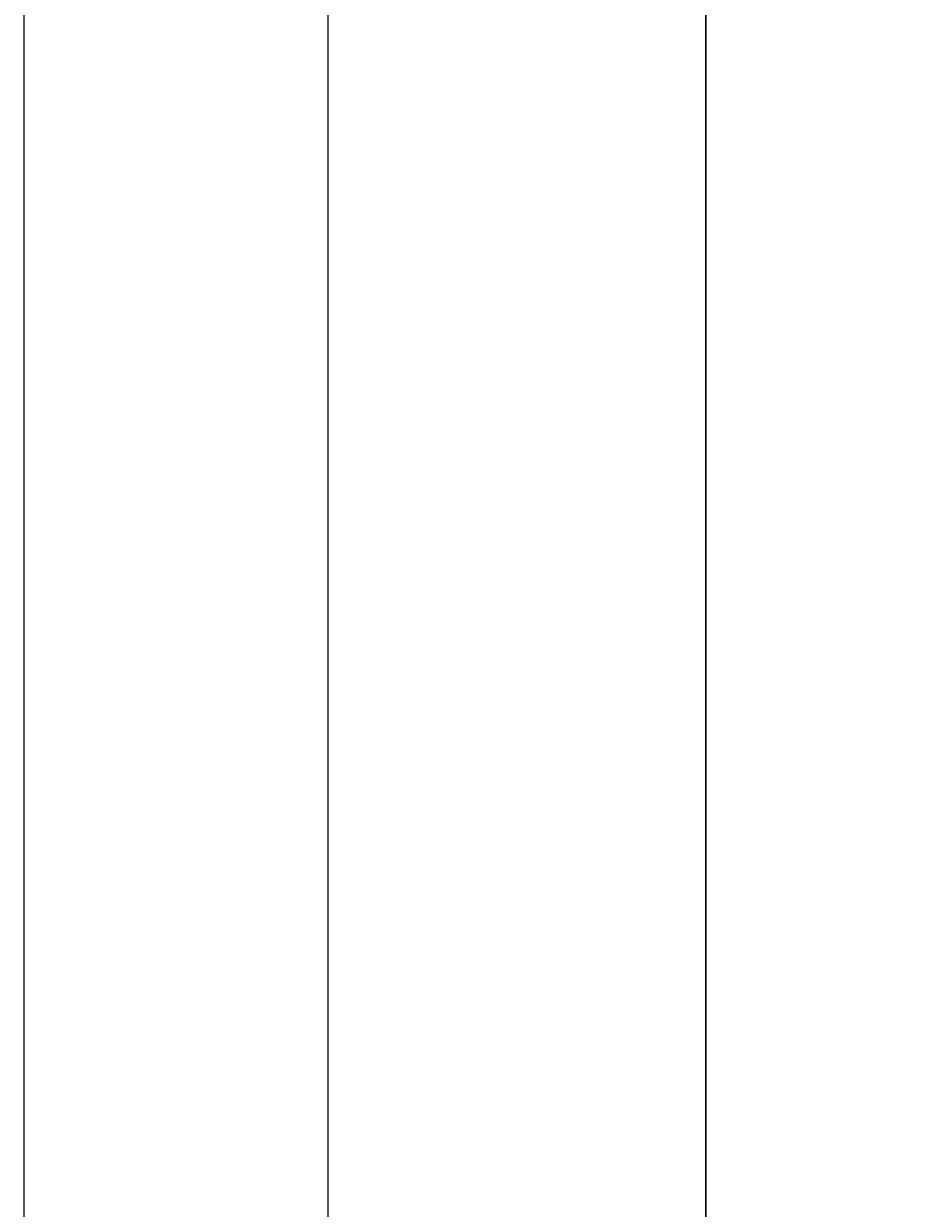
# Model space of a CAD drawing. Units: inches. Extents: x 2812 to 3051, y 1398 to 1659.
# Tile 28 of 65: x 2945 to 2966, y 1500 to 1528. Entities that reach past the tile are written whole.
import ezdxf

# ---------------------------------------------------------------- set-up
doc = ezdxf.new("R2010")
doc.units = ezdxf.units.IN
doc.layers.add('A-ANNO-DIMS', color=2, linetype='Continuous', lineweight=18)
doc.styles.get("Standard").update_dxf_attribs({"font": 'arial.ttf'})
doc.dimstyles.get("Standard").update_dxf_attribs({"dimtxt": 0.18, "dimasz": 0.18, "dimexe": 0.18, "dimexo": 0.0625, "dimgap": 0.09, "dimtad": 0, "dimtih": 1, "dimtoh": 1, "dimdec": 4, "dimzin": 0, "dimdsep": 46, "dimtxsty": 'Standard', "dimcen": 0.09, "dimadec": 0, "dimazin": 0, "dimtfac": 1, "dimtdec": 4, "dimtofl": 0, "dimtmove": 0, "dimatfit": 3, "dimfxl": 1, "dimtolj": 1, "dimtzin": 0, "dimarcsym": 0})

# ---------------------------------------------------------------- blocks, each defined once
blk = doc.blocks.new('*D30')
at = {"layer": 'A-ANNO-DIMS', "color": 0, "lineweight": -2, "transparency": 16777216}
for p, q in [((2945.147, 1598.692), (2945.147, 1397.505)), ((2952.385, 1559.757), (2952.385, 1397.505)), ((2945.327, 1397.685), (2948.373, 1397.685)), ((2952.205, 1397.685), (2949.159, 1397.685))]:
    blk.add_line(p, q, dxfattribs=at)
at = {"layer": 'A-ANNO-DIMS', "color": 0, "transparency": 16777216}
for points in [[(2945.327, 1397.715), (2945.327, 1397.655), (2945.147, 1397.685)], [(2952.205, 1397.715), (2952.205, 1397.655), (2952.385, 1397.685)]]:
    blk.add_solid(points, dxfattribs=at)
at = {"layer": 'Defpoints', "color": 0, "transparency": 16777216}
for p in [(2945.147, 1598.754), (2952.385, 1559.82), (2952.385, 1397.685)]:
    blk.add_point(p, dxfattribs=at)
at = {"layer": 'A-ANNO-DIMS', "color": 0, "transparency": 16777216, "insert": (2948.766, 1397.685), "char_height": 0.18, "attachment_point": 5}
blk.add_mtext('\\A1;7.238', dxfattribs=at)
blk = doc.blocks.new('*D31')
at = {"layer": 'A-ANNO-DIMS', "color": 0, "lineweight": -2, "transparency": 16777216}
for p, q in [((2972.272, 1594.192), (2972.272, 1397.505)), ((2961.385, 1559.757), (2961.385, 1397.505)), ((2961.565, 1397.685), (2966.373, 1397.685)), ((2972.092, 1397.685), (2967.283, 1397.685))]:
    blk.add_line(p, q, dxfattribs=at)
at = {"layer": 'A-ANNO-DIMS', "color": 0, "transparency": 16777216}
for points in [[(2961.565, 1397.715), (2961.565, 1397.655), (2961.385, 1397.685)], [(2972.092, 1397.715), (2972.092, 1397.655), (2972.272, 1397.685)]]:
    blk.add_solid(points, dxfattribs=at)
at = {"layer": 'Defpoints', "color": 0, "transparency": 16777216}
for p in [(2972.272, 1594.254), (2961.385, 1559.82), (2972.272, 1397.685)]:
    blk.add_point(p, dxfattribs=at)
at = {"layer": 'A-ANNO-DIMS', "color": 0, "transparency": 16777216, "insert": (2966.828, 1397.685), "char_height": 0.18, "attachment_point": 5}
blk.add_mtext('\\A1;10.887', dxfattribs=at)
blk = doc.blocks.new('*D69')
at = {"layer": 'A-ANNO-DIMS', "color": 0, "lineweight": -2, "transparency": 16777216}
for p, q in [((2961.385, 1472.098), (2961.385, 1659.35)), ((2968.956, 1467.81), (2968.956, 1659.35)), ((2961.565, 1659.17), (2964.795, 1659.17)), ((2968.776, 1659.17), (2965.546, 1659.17))]:
    blk.add_line(p, q, dxfattribs=at)
at = {"layer": 'A-ANNO-DIMS', "color": 0, "transparency": 16777216}
for points in [[(2961.565, 1659.2), (2961.565, 1659.14), (2961.385, 1659.17)], [(2968.776, 1659.2), (2968.776, 1659.14), (2968.956, 1659.17)]]:
    blk.add_solid(points, dxfattribs=at)
at = {"layer": 'Defpoints', "color": 0, "transparency": 16777216}
for p in [(2968.956, 1659.17), (2961.385, 1472.035), (2968.956, 1467.747)]:
    blk.add_point(p, dxfattribs=at)
at = {"layer": 'A-ANNO-DIMS', "color": 0, "transparency": 16777216, "insert": (2965.17, 1659.17), "char_height": 0.18, "attachment_point": 5}
blk.add_mtext('\\A1;7.571', dxfattribs=at)

msp = doc.modelspace()

# ---------------------------------------------------------------- dimensions: what is measured, and where the dimension line sits
at = {"layer": 'A-ANNO-DIMS'}
for base, p1, p2, picture, middle in [((2968.9558, 1659.17), (2961.3849, 1472.0354), (2968.9558, 1467.7474), '*D69', (2965.1704, 1659.17)), ((2952.3849, 1397.6854), (2945.1467, 1598.7541), (2952.3849, 1559.82), '*D30', (2948.7658, 1397.6854)), ((2972.2716, 1397.6854), (2961.3849, 1559.82), (2972.2716, 1594.2541), '*D31', (2966.8282, 1397.6854))]:
    dim = msp.add_linear_dim(base=base, p1=p1, p2=p2, dimstyle='Standard', override={"dimdec": 3, "dimlfac": 1, "dimrnd": 0, "dimzin": 0, "dimdsep": 46, "dimlunit": 2}, dxfattribs=at)
    dim.commit()
    dim.dimension.update_dxf_attribs({"geometry": picture, "text_midpoint": middle})

doc.saveas('drawing.dxf')
